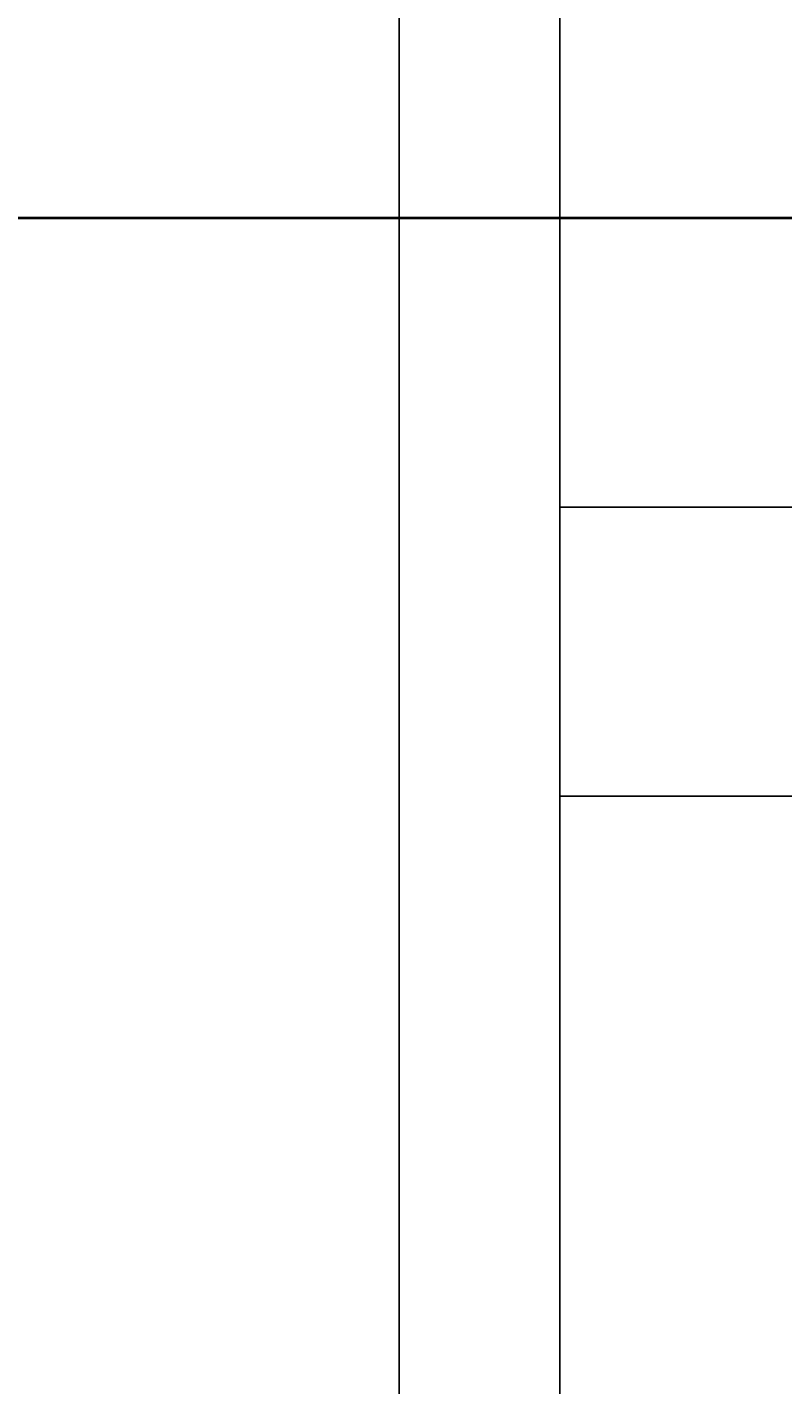
# Model space of a CAD drawing. Units: inches. Extents: x -301 to 715, y -607 to 364.
# Tile 64 of 141: x -62 to -39, y -260 to -218. Entities that reach past the tile are written whole.
import ezdxf

# ---------------------------------------------------------------- set-up
doc = ezdxf.new("R2010")
doc.units = ezdxf.units.IN
doc.header["$MEASUREMENT"] = 0
for name, color, linetype, lineweight in [('A-ANNO-DIMS', 2, 'Continuous', 18), ('A-FLOR-STRS', 2, 'Continuous', 25), ('A-WALL', 3, 'Continuous', 40)]:
    doc.layers.add(name, color=color, linetype=linetype, lineweight=lineweight)
doc.styles.get("Standard").update_dxf_attribs({"font": 'arial.ttf'})
doc.dimstyles.get("Standard").update_dxf_attribs({"dimtxt": 0.18, "dimasz": 0.18, "dimexe": 0.18, "dimexo": 0.0625, "dimgap": 0.09, "dimtad": 0, "dimtih": 1, "dimtoh": 1, "dimdec": 1, "dimzin": 0, "dimdsep": 46, "dimlunit": 4, "dimtxsty": 'Standard', "dimcen": 0.09, "dimclrd": 3, "dimclre": 4, "dimclrt": 6, "dimadec": 0, "dimazin": 0, "dimtfac": 1, "dimtdec": 1, "dimtofl": 0, "dimtmove": 0, "dimatfit": 3, "dimfxl": 1, "dimtfill": 2, "dimtfillclr": 51, "dimtolj": 1, "dimtzin": 0, "dimarcsym": 0})

# ---------------------------------------------------------------- blocks, each defined once
blk = doc.blocks.new('ENTRY-STEPS-48')
for p, q in [((0, 27), (0, 18)), ((48, 27), (48, 18)), ((0, 18), (0, 9)), ((48, 9), (48, 18)), ((0, 9), (48, 9)), ((0, 9), (0, 0)), ((48, 0), (48, 9)), ((0, 0), (48, 0))]:
    blk.add_line(p, q)
blk = doc.blocks.new('*D147')
at = {"layer": 'A-ANNO-DIMS', "color": 4, "lineweight": -2, "transparency": 16777216}
for p, q in [((-103.603, -223.88), (-103.603, -296.865)), ((-45.603, -223.88), (-45.603, -296.865))]:
    blk.add_line(p, q, dxfattribs=at)
at = {"layer": 'A-ANNO-DIMS', "color": 3, "lineweight": -2, "transparency": 16777216}
for p, q in [((-103.423, -296.685), (-75.006, -296.685)), ((-45.783, -296.685), (-74.2, -296.685))]:
    blk.add_line(p, q, dxfattribs=at)
at = {"layer": 'A-ANNO-DIMS', "color": 3, "transparency": 16777216}
for points in [[(-103.423, -296.655), (-103.423, -296.715), (-103.603, -296.685)], [(-45.783, -296.655), (-45.783, -296.715), (-45.603, -296.685)]]:
    blk.add_solid(points, dxfattribs=at)
at = {"layer": 'Defpoints', "color": 0, "transparency": 16777216}
for p in [(-103.603, -223.818), (-45.603, -223.818), (-45.603, -296.685)]:
    blk.add_point(p, dxfattribs=at)
at = {"layer": 'A-ANNO-DIMS', "color": 6, "transparency": 16777216, "insert": (-74.603, -296.685), "char_height": 0.18, "attachment_point": 5, "bg_fill": 1, "box_fill_scale": 1.25, "bg_fill_color": 51, "bg_fill_transparency": 0}
blk.add_mtext('\\A1;4\'-10"', dxfattribs=at)
blk = doc.blocks.new('*D151')
at = {"layer": 'A-ANNO-DIMS', "color": 4, "lineweight": -2, "transparency": 16777216}
for p, q in [((-204.603, -223.755), (-204.603, 359.612)), ((-45.603, -214.755), (-45.603, 359.612))]:
    blk.add_line(p, q, dxfattribs=at)
at = {"layer": 'A-ANNO-DIMS', "color": 3, "lineweight": -2, "transparency": 16777216}
for p, q in [((-204.423, 359.432), (-125.494, 359.432)), ((-45.783, 359.432), (-124.713, 359.432))]:
    blk.add_line(p, q, dxfattribs=at)
at = {"layer": 'A-ANNO-DIMS', "color": 3, "transparency": 16777216}
for points in [[(-204.423, 359.462), (-204.423, 359.402), (-204.603, 359.432)], [(-45.783, 359.462), (-45.783, 359.402), (-45.603, 359.432)]]:
    blk.add_solid(points, dxfattribs=at)
at = {"layer": 'Defpoints', "color": 0, "transparency": 16777216}
for p in [(-45.603, 359.432), (-45.603, -214.818), (-204.603, -223.818)]:
    blk.add_point(p, dxfattribs=at)
at = {"layer": 'A-ANNO-DIMS', "color": 6, "transparency": 16777216, "insert": (-125.103, 359.432), "char_height": 0.18, "attachment_point": 5, "bg_fill": 1, "box_fill_scale": 1.25, "bg_fill_color": 51, "bg_fill_transparency": 0}
blk.add_mtext('\\A1;13\'-3"', dxfattribs=at)
blk = doc.blocks.new('*D158')
at = {"layer": 'A-ANNO-DIMS', "color": 4, "lineweight": -2, "transparency": 16777216}
for p, q in [((-122.603, 221.62), (-122.603, -296.865)), ((-50.603, 221.62), (-50.603, -296.865))]:
    blk.add_line(p, q, dxfattribs=at)
at = {"layer": 'A-ANNO-DIMS', "color": 3, "lineweight": -2, "transparency": 16777216}
for p, q in [((-122.423, -296.685), (-86.933, -296.685)), ((-50.783, -296.685), (-86.274, -296.685))]:
    blk.add_line(p, q, dxfattribs=at)
at = {"layer": 'A-ANNO-DIMS', "color": 3, "transparency": 16777216}
for points in [[(-122.423, -296.655), (-122.423, -296.715), (-122.603, -296.685)], [(-50.783, -296.655), (-50.783, -296.715), (-50.603, -296.685)]]:
    blk.add_solid(points, dxfattribs=at)
at = {"layer": 'Defpoints', "color": 0, "transparency": 16777216}
for p in [(-122.603, 221.682), (-50.603, 221.682), (-50.603, -296.685)]:
    blk.add_point(p, dxfattribs=at)
at = {"layer": 'A-ANNO-DIMS', "color": 6, "transparency": 16777216, "insert": (-86.603, -296.685), "char_height": 0.18, "attachment_point": 5, "bg_fill": 1, "box_fill_scale": 1.25, "bg_fill_color": 51, "bg_fill_transparency": 0}
blk.add_mtext('\\A1;6\'-0"', dxfattribs=at)

msp = doc.modelspace()

# ---------------------------------------------------------------- linework, layer by layer
at = {"layer": 'A-WALL'}
for p, q in [((-204.603, -223.818), (-45.603, -223.818)), ((-45.603, -223.818), (132.897, -223.818))]:
    msp.add_line(p, q, dxfattribs=at)

# ---------------------------------------------------------------- block references
at = {"layer": 'A-FLOR-STRS'}
msp.add_blockref('ENTRY-STEPS-48', (-45.603, -241.818), dxfattribs=at)

# ---------------------------------------------------------------- dimensions: what is measured, and where the dimension line sits
at = {"layer": 'A-ANNO-DIMS'}
for base, p1, p2, picture, middle in [((-45.603, 359.432), (-204.603, -223.818), (-45.603, -214.818), '*D151', (-125.103, 359.432)), ((-50.603, -296.685), (-122.603, 221.682), (-50.603, 221.682), '*D158', (-86.603, -296.685)), ((-45.603, -296.685), (-103.603, -223.818), (-45.603, -223.818), '*D147', (-74.603, -296.685))]:
    dim = msp.add_linear_dim(base=base, p1=p1, p2=p2, dimstyle='Standard', override={"dimdec": 1, "dimlfac": 1, "dimrnd": 0, "dimzin": 1, "dimdsep": 46, "dimlunit": 4, "dimfrac": 2}, dxfattribs=at)
    dim.commit()
    dim.dimension.update_dxf_attribs({"geometry": picture, "text_midpoint": middle})

doc.saveas('drawing.dxf')
